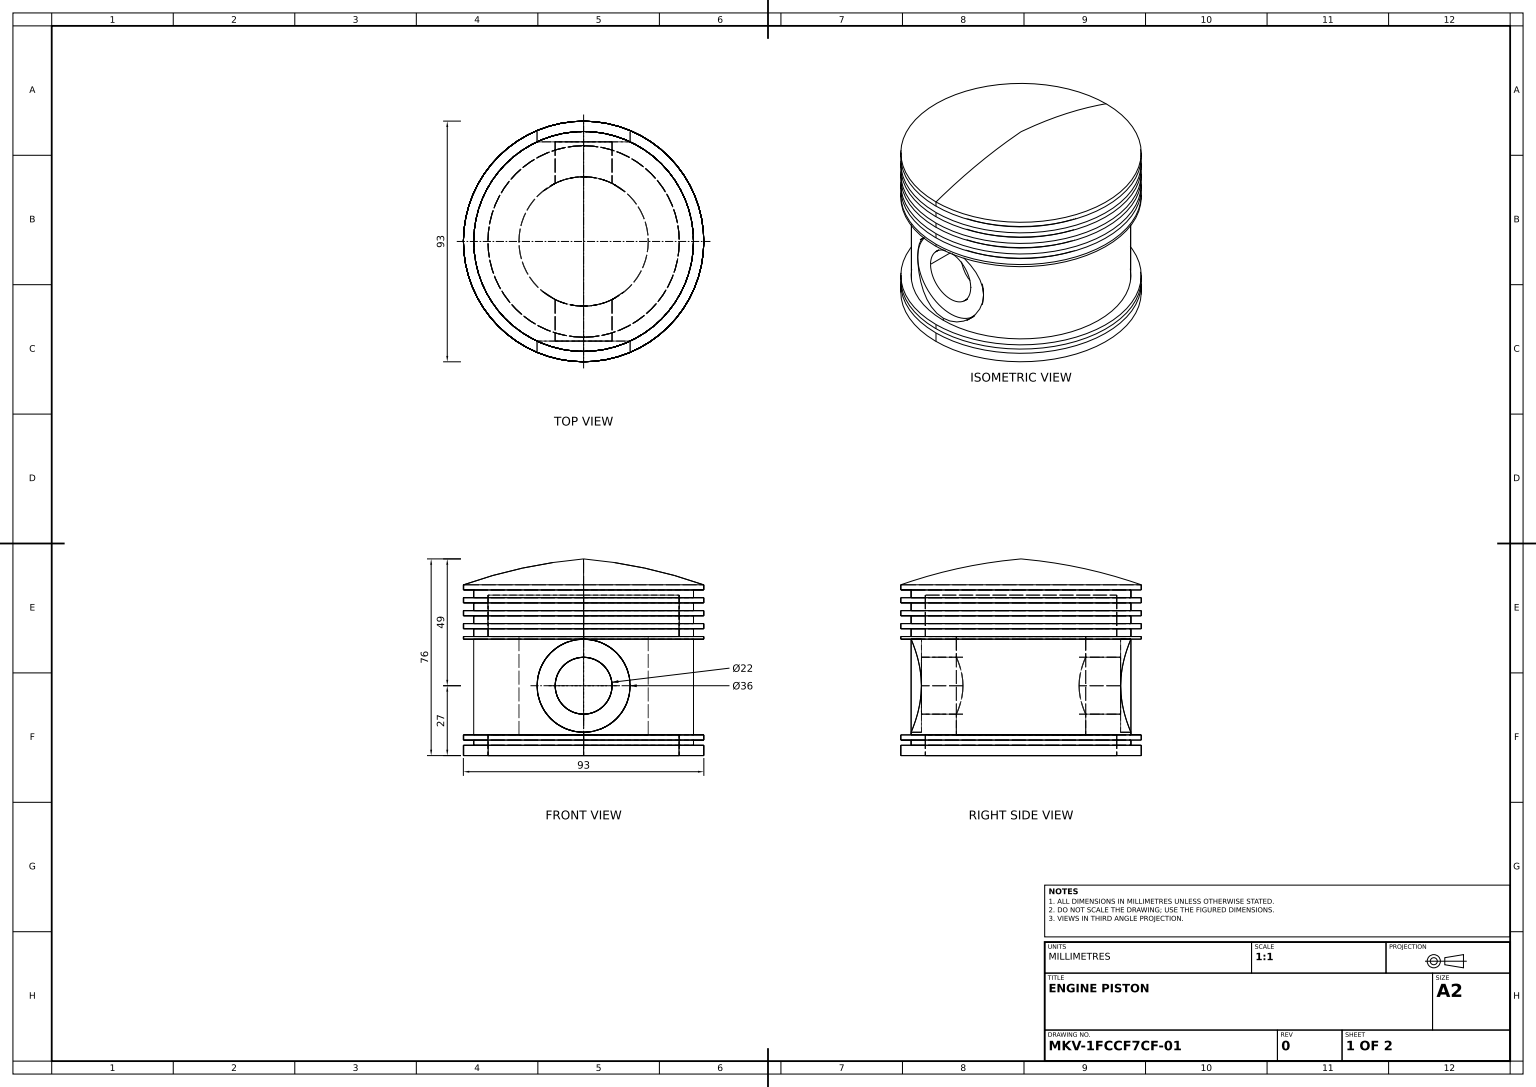
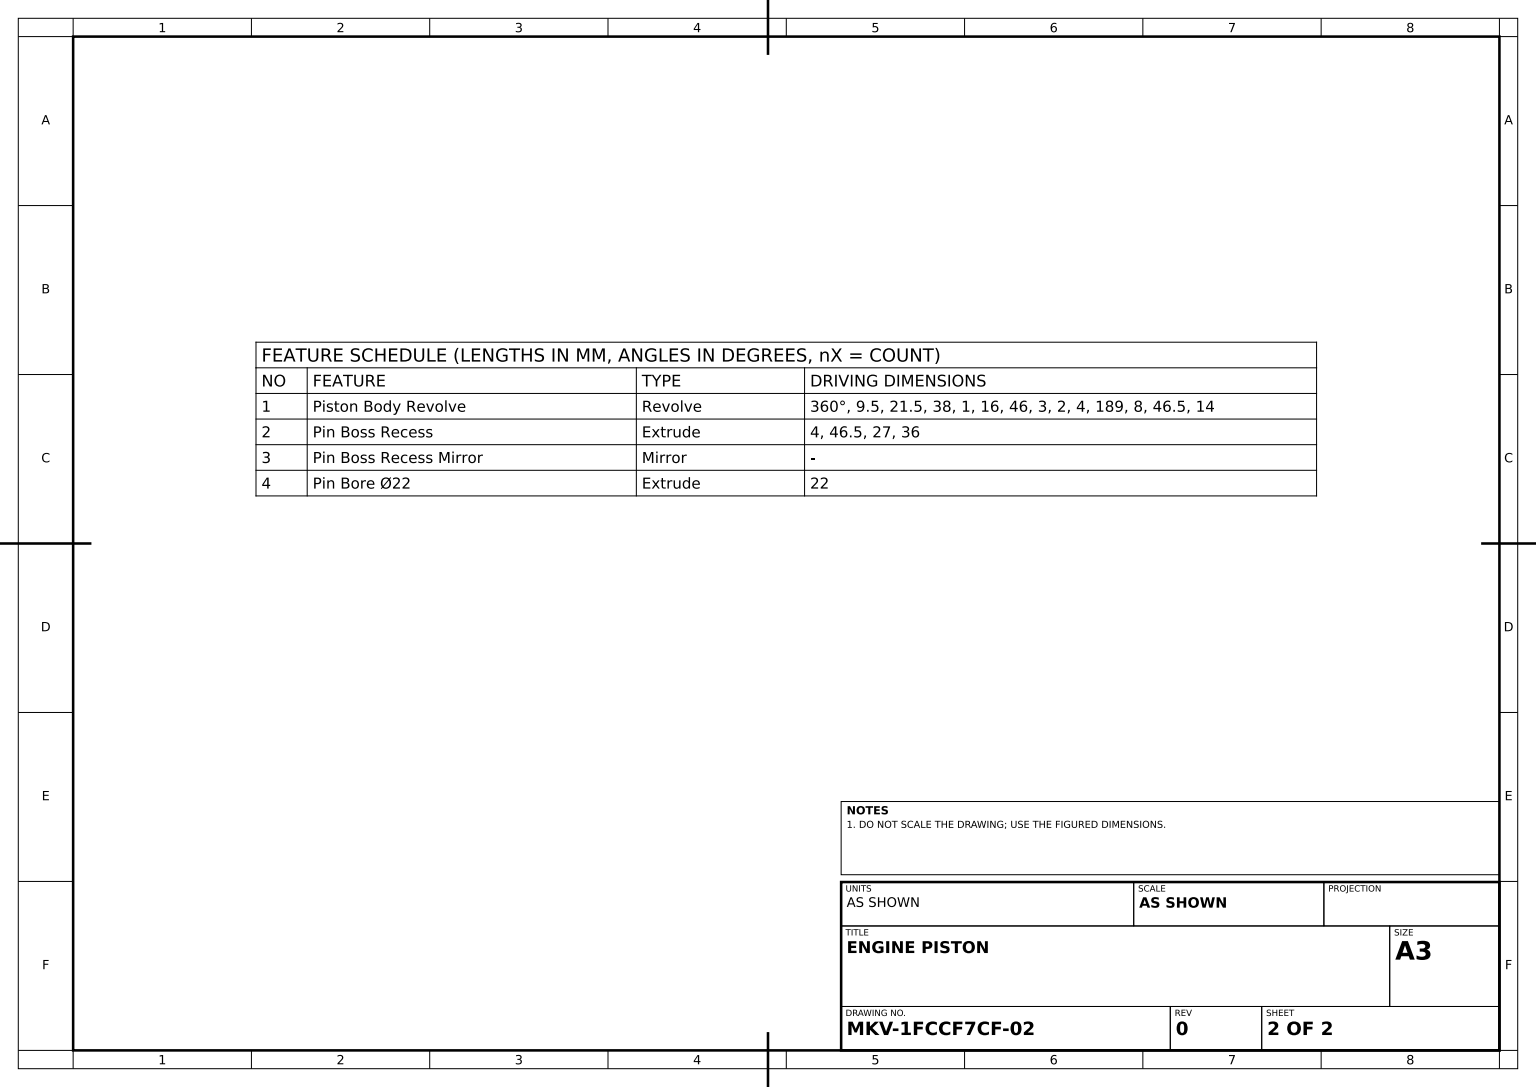
SolidWorks part; units mm, degrees
material "Plain Carbon Steel"
ref_plane "Front Plane" through (0, 0, 0) normal (0, 0, 1) x (1, 0, 0)
ref_plane "Top Plane" through (0, 0, 0) normal (0, 1, 0) x (1, 0, 0)
ref_plane "Right Plane" through (0, 0, 0) normal (1, 0, 0) x (0, 0, -1)
sketch "Piston Profile Sketch" plane through (0, 0, 0) normal (0, 0, 1) x (1, 0, 0)
  line L0 (0, 0) -> (9.5, 0)
  line L1 (9.5, 0) -> (9.5, 8)
  line L2 (9.5, 8) -> (21.5, 8)
  line L3 (21.5, 8) -> (21.5, 46)
  line L4 (21.5, 46) -> (9.5, 46)
  line L5 (9.5, 46) -> (9.5, 62)
  line L6 (9.5, 62) -> (46.5, 62)
  line L9 (0, 66) -> (0, 64)
  line L10 (46.5, 62) -> (46.5, 76)
  line L11 (0, 61) -> (4, 61)
  line L12 (0, 51) -> (4, 51)
  line L13 (0, 56) -> (4, 56)
  line L14 (0, 54) -> (4, 54)
  line L15 (0, 64) -> (4, 64)
  line L16 (0, 46) -> (4, 46)
  line L17 (0, 49) -> (4, 49)
  line L18 (0, 45) -> (4, 45)
  line L19 (0, 59) -> (4, 59)
  line L20 (0, 4) -> (4, 4)
  line L21 (0, 8) -> (4, 8)
  line L22 (0, 6) -> (4, 6)
  line L23 (4, 45) -> (4, 8)
  line L24 (0, 46) -> (0, 45)
  line L25 (4, 49) -> (4, 46)
  line L26 (0, 51) -> (0, 49)
  line L27 (4, 54) -> (4, 51)
  line L28 (0, 56) -> (0, 54)
  line L30 (4, 59) -> (4, 56)
  line L31 (0, 61) -> (0, 59)
  line L32 (4, 64) -> (4, 61)
  line L33 (0, 4) -> (0, 0)
  line L34 (4, 6) -> (4, 4)
  line L35 (0, 8) -> (0, 6)
  line L36 (46.5, 0) -> (46.5, 13.17) construction
  arc A1 (0, 66) -> (46.5, 76) centre (62.6708, -112.3069) cw
  dimension "D22" = 189
  dimension "D23" = 46.5
  dimension "D1" = 9.5
  dimension "D3" = 21.5
  dimension "D4" = 0
  dimension "D5" = 38
  dimension "D6" = 1
  dimension "D7" = 16
  dimension "D8" = 4
  dimension "D9" = 62
  dimension "D10" = 46
  dimension "D11" = 8
  dimension "D12" = 3
  dimension "D13" = 2
  dimension "D14" = 3
  dimension "D15" = 2
  dimension "D16" = 3
  dimension "D17" = 2
  dimension "D18" = 3
  dimension "D19" = 4
  dimension "D20" = 2
  dimension "D21" = 2
  dimension "D24" = 14
  dimension "D25" = 2
revolve "Piston Body Revolve" add sketch "Piston Profile Sketch" angle 360 about L36
ref_plane "Plane3" through (89, 0, 0) normal (1, 0, 0) x (0, 0, -1)
ref_plane "Pin Boss Plane" through (0, 0, 42.5) normal (0, 0, 1) x (1, 0, 0)
sketch "Pin Boss Recess Sketch" plane through (0, 0, 42.5) normal (0, 0, 1) x (1, 0, 0)
  line L0 (0, 0) -> (93, 0) construction
  circle A0 centre (46.5, 27) radius 18
  dimension "D3" = 36
  dimension "D1" = 46.5
  dimension "D2" = 27
extrude "Pin Boss Recess" cut sketch "Pin Boss Recess Sketch" against normal blind 4
mirror "Pin Boss Recess Mirror" about plane through (0, 0, 0) normal (0, 0, 1) of "Pin Boss Recess"
sketch "Pin Bore Sketch" plane through (0, 0, 42.5) normal (0, 0, 1) x (1, 0, 0)
  circle A0 centre (46.5, 27) radius 11
  dimension "D1" = 22
extrude "Pin Bore Ø22" cut sketch "Pin Bore Sketch" against normal through all
